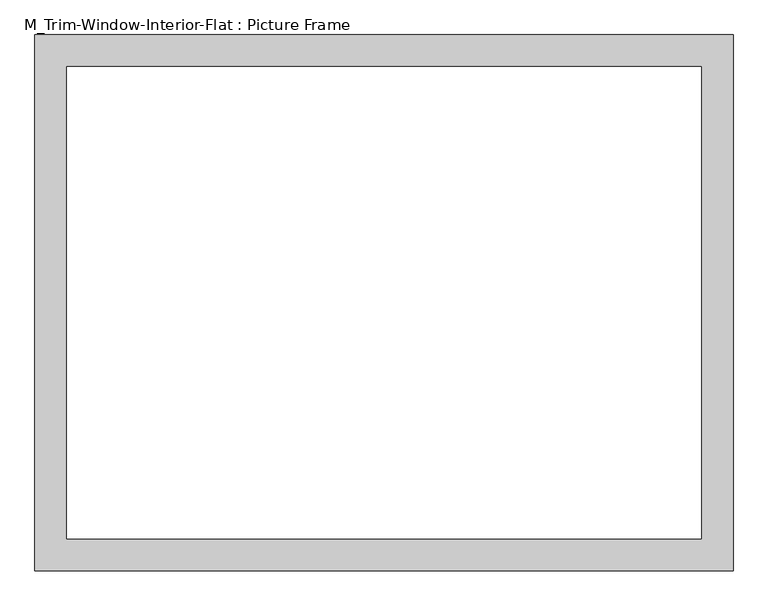
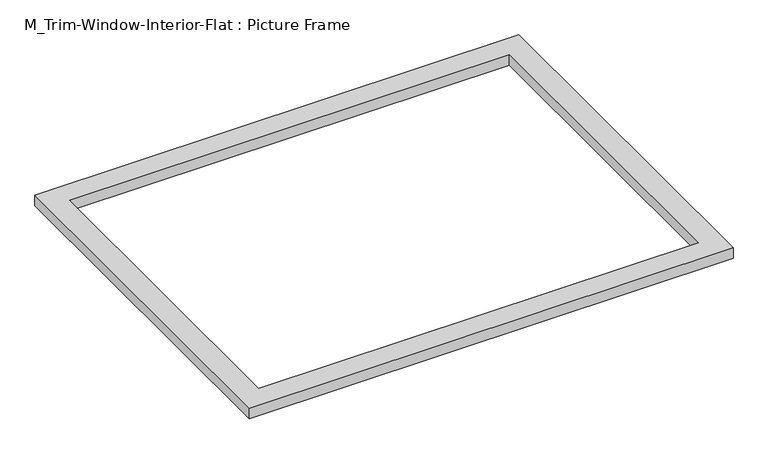
"""IFC4 building model written with IfcOpenShell, lengths in millimetres: proxy geometry, M_Trim-Window-Interior-Flat : Picture Frame."""

from ifc_helpers import new_model, si_unit, origin, origin_with_axes, place, context, project, spatial, polyline, outline, extrude, source, transform, mapped, element, save


def m_trim_window_interior_flat_picture_frame_fffd0b6f(model_context):
    return source(origin(), model_context, "Body", "SweptSolid", [
        extrude(outline(polyline([(656.9, 47.3), (656.9, -961.7), (-656.9, -961.7), (-656.9, 47.3), (656.9, 47.3)]), holes=[polyline([(596.9, -12.7), (-596.9, -12.7), (-596.9, -901.7), (596.9, -901.7), (596.9, -12.7)])]), origin_with_axes(), (0.0, 0.0, 1.0), 30.0),
    ])


if __name__ == "__main__":
    model = new_model("IFC4")
    model_context = context("Model", 3, world=origin())
    ifc_project = project(units=[si_unit("LENGTHUNIT", "METRE", prefix="MILLI")], contexts=[model_context])
    site = spatial("IfcSite", under=ifc_project)
    building = spatial("IfcBuilding", under=site)
    placement = place(None, origin())
    m_trim_window_interior_flat_picture_frame_shape = m_trim_window_interior_flat_picture_frame_fffd0b6f(model_context)
    element("IfcBuildingElementProxy", 1, Name="M_Trim-Window-Interior-Flat : Picture Frame", ObjectType="M_Trim-Window-Interior-Flat : Picture Frame", at=placement, inside=building, context=model_context, shape_type="MappedRepresentation", body=[
        mapped(m_trim_window_interior_flat_picture_frame_shape, transform((0.0, 0.0, 0.0), x_axis=(1.0, 0.0, 0.0), y_axis=(0.0, 1.0, 0.0), z_axis=(0.0, 0.0, 1.0))),
    ])
    save(model, "model.ifc")

# Revit data of these elements
# Type "M_Trim-Window-Interior-Flat : Picture Frame"
#   Trim Thickness_Picture Frame = 0' - 1.1811"
#   Trim Width = 0' - 2.3622"
#   Trim Thickness_with Sill = 0' - 0.7874"
#   Sill Thickness = 0' - 1.1811"
#   Opening Width [instance default] = 1' - 11.62205"
#   Opening Height [instance default] = 2' - 11.43307"
#   Default Elevation = 3' - 11.24409"
#   Sill = no
#   Picture Frame = yes
#   Trim Material [instance default] = none
# Element 1 (IfcBuildingElementProxy, "M_Trim-Window-Interior-Flat : Picture Frame")
#   Opening Width = 4' - 0"
#   Opening Height = 3' - 0"
#   Trim Material = Wood - Stained
#   Materials on its faces: "Wood - Stained"
# Materials
#   "Wood - Stained": class "Wood", colour RGB 224 178 126, transparency 0, Cost = 0
